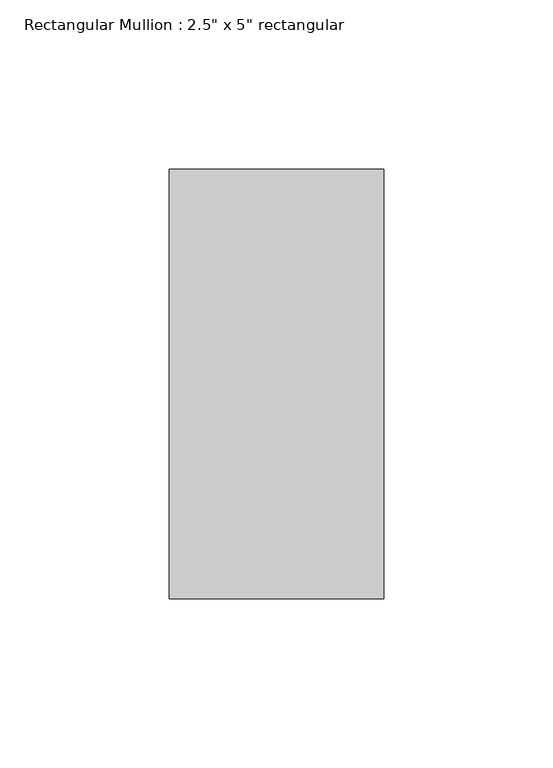
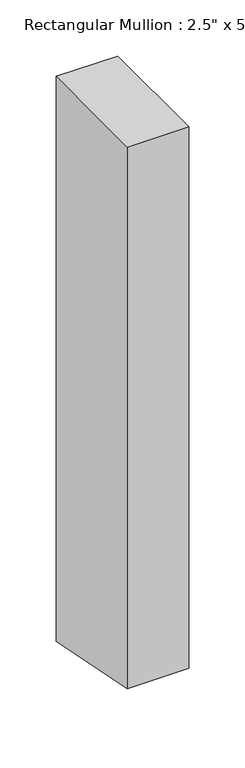
"""IFC4 building model written with IfcOpenShell, lengths in millimetres: member geometry."""

from ifc_helpers import new_model, si_unit, frame, origin, place, context, project, spatial, polyline, outline, extrude, source, transform, mapped, element, save


def member_6051e8ad(model_context):
    return source(origin(), model_context, "Body", "SweptSolid", [
        extrude(outline(polyline([(-63.5, 0.0), (63.5, 0.0), (63.5, -615.5583104), (-63.5, -590.2964398), (-63.5, 0.0)])), frame((-63.5, 0.0, 0.0), z_axis=(1.0, 0.0, 0.0), x_axis=(0.0, 1.0, 0.0)), (0.0, 0.0, 1.0), 63.5),
    ])


if __name__ == "__main__":
    model = new_model("IFC4")
    model_context = context("Model", 3, world=origin())
    ifc_project = project(units=[si_unit("LENGTHUNIT", "METRE", prefix="MILLI")], contexts=[model_context])
    site = spatial("IfcSite", under=ifc_project)
    building = spatial("IfcBuilding", under=site)
    placement = place(None, origin())
    member_shape = member_6051e8ad(model_context)
    element("IfcMember", 1, ObjectType="Rectangular Mullion : 2.5\" x 5\" rectangular", at=placement, inside=building, context=model_context, shape_type="MappedRepresentation", body=[
        mapped(member_shape, transform((0.0, 0.0, 0.0), x_axis=(1.0, 0.0, 0.0), y_axis=(0.0, 1.0, 0.0), z_axis=(0.0, 0.0, 1.0))),
    ])
    save(model, "model.ifc")

# Revit data of these elements
# Type "Rectangular Mullion : 2.5\" x 5\" rectangular"
#   built-in parameter 1007304 = 0.416667 (stored number, unit not read)
#   built-in parameter 1007301 = 0.104167 (stored number, unit not read)
#   built-in parameter 1007300 = 0.104167 (stored number, unit not read)
# Element 1 (IfcMember, "Rectangular Mullion : 2.5\" x 5\" rectangular")
#   Materials on its faces: "Iron, Ductile"
# Materials
#   "Iron, Ductile": class "Metal", colour RGB 0 0 0, transparency 0, Description = "Ductile cast iron", Cost = 0
